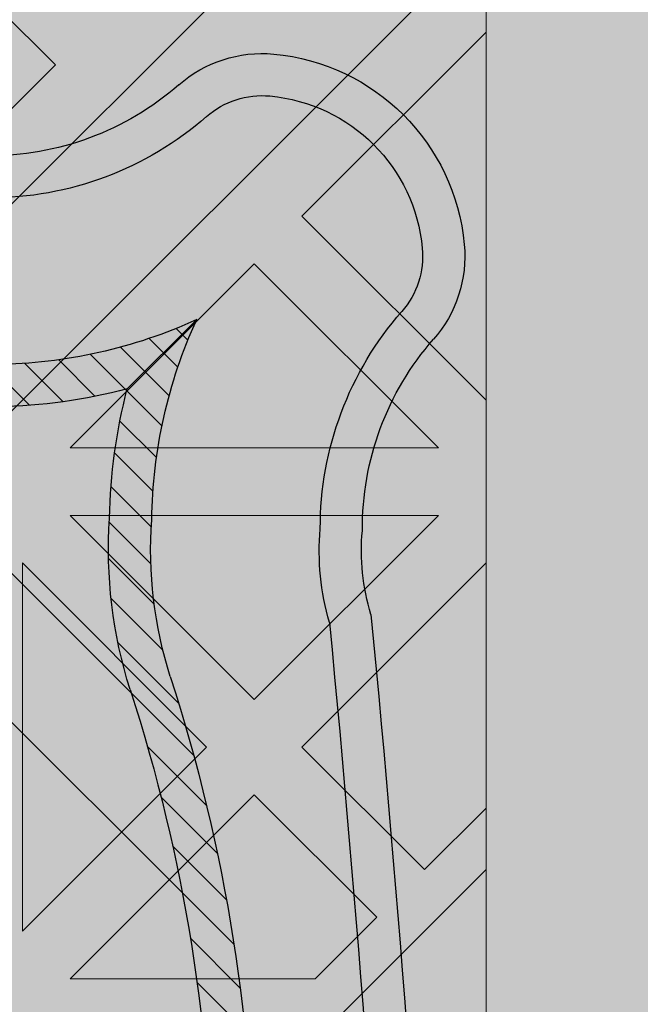
# Model space of a CAD drawing. Units: inches. Extents: x 844 to 2234, y 346 to 1084.
# Tile 39 of 93: x 1260.074 to 1262.421, y 701.353 to 705.079. Entities that reach past the tile are written whole.
import ezdxf

# ---------------------------------------------------------------- set-up
doc = ezdxf.new("R2010")
doc.units = ezdxf.units.IN
doc.header["$MEASUREMENT"] = 0
doc.layers.add('furniture', color=8, linetype='Continuous', lineweight=18)
doc.layers.add('RA-AP-01$0$INT', color=35, linetype='Continuous', lineweight=5)
doc.layers.add('RA-AP-01$0$FURN', color=3, linetype='Continuous')
doc.layers.add('RA-AP-01$0$WOOD', color=64, linetype='Continuous')

# ---------------------------------------------------------------- blocks, each defined once
blk = doc.blocks.new('A$C18D01794')
at = {"layer": 'RA-AP-01$0$INT'}
blk.add_hatch(color=256, dxfattribs=at).paths.add_polyline_path([(4.505206456958071, -7.906712009588039), (5.305206456958072, -7.906712009588039), (5.305206456958072, -7.106712009588038), (5.255206456951893, -7.106712009588036), (5.25520645694868, -7.856712009570104), (4.555206456959269, -7.856712009588616), (4.555206456956052, -7.106712009588038), (4.505206456958073, -7.106712009588038)])
h = blk.add_hatch(color=256, dxfattribs=at)
h.paths.add_polyline_path([(4.585917135068448, -7.856712009587804), (4.614201406330596, -7.856712009587056), (4.668846067270487, -7.802067348644738), (4.723490728212344, -7.856712009584164), (4.771774999457151, -7.856712009582887), (4.826419660396886, -7.80206734864072), (4.862780050090322, -7.838427738332541), (4.844495778842715, -7.856712009580965), (4.862780050090411, -7.856712009580482), (4.905206456960182, -7.814285602707865), (4.947632863832445, -7.856712009578238), (4.965917135079675, -7.856712009577755), (4.947632863831759, -7.838427738330656), (4.983993253523576, -7.802067348637219), (5.038637914464627, -7.856712009575829), (5.08692218571208, -7.856712009574554), (5.141566846649976, -7.802067348634224), (5.196211507589851, -7.856712009571666), (5.224495778822615, -7.856712009570916), (4.905206456953975, -7.537422687702283)])
h.paths.add_polyline_path([(4.895206456956031, -7.575706958950402), (4.895206456958921, -7.684996280828174), (4.840561796018589, -7.630351619890275)], flags=16)
h.paths.add_polyline_path([(4.915206456955638, -7.575706958949956), (4.969851117895509, -7.630351619887399), (4.915206456957609, -7.684996280827732)], flags=16)
h.paths.add_polyline_path([(4.826419660395175, -7.644493755514321), (4.881064321335613, -7.699138416452331), (4.771774999456703, -7.69913841645522)], flags=16)
h.paths.add_polyline_path([(4.983993253519558, -7.644493755510815), (5.038637914460456, -7.699138416449285), (4.929348592581548, -7.69913841645126)], flags=16)
h.paths.add_polyline_path([(4.881064321336025, -7.719138416452334), (4.826419660397532, -7.773783077393256), (4.771774999457062, -7.719138416455217)], flags=16)
h.paths.add_polyline_path([(4.929348592582019, -7.71913841645126), (5.038637914460982, -7.719138416449284), (4.983993253522945, -7.773783077389749)], flags=16)
h.paths.add_polyline_path([(4.895206456960191, -7.733280552075633), (4.895206456962115, -7.806001331460164), (4.876922185715016, -7.824285602708492), (4.840561796021581, -7.787925213016675)], flags=16)
h.paths.add_polyline_path([(4.915206456958487, -7.733280552075187), (4.969851117899527, -7.787925213013798), (4.933490728206909, -7.824285602708034), (4.9152064569598, -7.806001331461736)], flags=16)
h.paths.add_polyline_path([(4.757632863832376, -7.733280552079264), (4.812277524772842, -7.787925213017304), (4.757632863834348, -7.842569873958233)], flags=16)
h.paths.add_polyline_path([(4.737632863832376, -7.73328055207979), (4.737632863834348, -7.842569873958701), (4.682988202893906, -7.787925213020692)], flags=16)
h.paths.add_polyline_path([(5.05278005008503, -7.733280552072701), (5.052780050087917, -7.842569873951664), (4.998135389146995, -7.787925213013169)], flags=16)
h.paths.add_polyline_path([(5.072780050085024, -7.733280552072333), (5.127424711025931, -7.787925213010806), (5.072780050087916, -7.842569873951244)], flags=16)
h.paths.add_polyline_path([(4.935917135072783, -7.506712009583784), (5.255206456948811, -7.826001331459767), (5.255206456948932, -7.797717060211899), (5.200561796010279, -7.743072399273238), (5.255206456949403, -7.688427738334128), (5.25520645694961, -7.640143467086677), (5.200561796009787, -7.585498806146837), (5.236922185702417, -7.549138416454212), (5.255206456949919, -7.56742268770172), (5.255206456949998, -7.549138416454178), (5.212780050078687, -7.506712009583814), (5.25520645695036, -7.464285602712145), (5.255206456950438, -7.446001331464763), (5.236922185702424, -7.464285602712779), (5.200561796009796, -7.427925213020149), (5.255206456950753, -7.373280552079203), (5.25520645695096, -7.324996280834394), (5.200561796010322, -7.270351619893748), (5.255206456951428, -7.215706958952649), (5.255206456951547, -7.187422687705071)])
h.paths.add_polyline_path([(5.042988202883395, -7.42792521302065), (5.097632863823085, -7.373280552080975), (5.097632863822622, -7.482569873959883)], flags=16)
h.paths.add_polyline_path([(5.028846067259663, -7.442067348644384), (5.083490728198774, -7.496712009583504), (4.974201406321001, -7.496712009583035)], flags=16)
h.paths.add_polyline_path([(5.117632863823087, -7.37328055208089), (5.172277524762331, -7.42792521302015), (5.11763286382262, -7.482569873959851)], flags=16)
h.paths.add_polyline_path([(5.08349072819877, -7.516712009582191), (5.028846067259652, -7.571356670521302), (4.974201406320998, -7.516712009582638)], flags=16)
h.paths.add_polyline_path([(5.131774999446817, -7.35913841645716), (5.186419660386065, -7.413783077396415), (5.241064321325782, -7.359138416456712)], flags=17)
h.paths.add_polyline_path([(5.131774999446228, -7.496712009583703), (5.186419660386065, -7.442067348643883), (5.222780050079488, -7.478427738337313), (5.204495778832781, -7.496712009584014)], flags=16)
h.paths.add_polyline_path([(5.097632863822613, -7.530854145205813), (5.097632863823061, -7.640143467084723), (5.042988202883383, -7.585498806145032)], flags=16)
h.paths.add_polyline_path([(5.131774999446899, -7.339138416457162), (5.241064321325809, -7.339138416456712), (5.186419660386591, -7.284493755517479)], flags=17)
h.paths.add_polyline_path([(5.131774999446226, -7.516712009581999), (5.204495778830767, -7.516712009581702), (5.22278005007868, -7.534996280829206), (5.186419660386049, -7.571356670521828)], flags=16)
h.paths.add_polyline_path([(5.11763286382262, -7.530854145205852), (5.17227752476232, -7.585498806145562), (5.117632863823064, -7.64014346708481)], flags=16)
h.paths.add_polyline_path([(5.186419660386069, -7.599640941770585), (5.241064321325754, -7.654285602710281), (5.131774999446791, -7.654285602709814)], flags=16)
h.paths.add_polyline_path([(5.131774999446872, -7.674285602709813), (5.24106432132578, -7.674285602710282), (5.186419660386554, -7.728930263649504)], flags=16)
h.paths.add_polyline_path([(5.255206456951811, -7.126001331467467), (5.255206456951895, -7.106712009588038), (4.555206456956052, -7.106712009588038), (4.555206456956136, -7.12600133146746), (4.905206456953973, -7.476001331465289)])
h.paths.add_polyline_path([(4.983993253513404, -7.368930263651977), (4.92934859257295, -7.314285602713969), (5.03863791445186, -7.314285602711063)], flags=16)
h.paths.add_polyline_path([(4.969851117889988, -7.383072399276016), (4.915206456952556, -7.437717060215906), (4.915206456949648, -7.328427738338133)], flags=16)
h.paths.add_polyline_path([(4.929348592572535, -7.294285602713971), (4.983993253511019, -7.239640941773039), (5.038637914451496, -7.294285602711065)], flags=16)
h.paths.add_polyline_path([(5.052780050074912, -7.280143467087016), (4.998135389134438, -7.225498806148989), (5.052780050072919, -7.170854145208052)], flags=16)
h.paths.add_polyline_path([(5.07278005007491, -7.280143467086489), (5.072780050072918, -7.170854145207579), (5.127424711013374, -7.225498806145578)], flags=16)
h.paths.add_polyline_path([(4.89520645695295, -7.437717060216355), (4.840561796013067, -7.383072399278919), (4.895206456950961, -7.328427738338582)], flags=16)
h.paths.add_polyline_path([(4.915206456948365, -7.280143467090674), (4.915206456946434, -7.207422687704125), (4.933490728192729, -7.18913841645701), (4.969851117886972, -7.225498806149623)], flags=16)
h.paths.add_polyline_path([(4.881064321327021, -7.314285602715054), (4.82641966038902, -7.368930263655506), (4.771774999448108, -7.314285602717047)], flags=16)
h.paths.add_polyline_path([(4.895206456950073, -7.280143467091125), (4.840561796009022, -7.225498806152518), (4.876922185700835, -7.18913841645908), (4.895206456948749, -7.207422687706589)], flags=16)
h.paths.add_polyline_path([(4.983993253510392, -7.211356670525576), (4.947632863816944, -7.174996280833758), (4.965917135064043, -7.156712009585847), (5.038637914448995, -7.156712009584522)], flags=16)
h.paths.add_polyline_path([(4.881064321326543, -7.294285602715056), (4.771774999447578, -7.294285602717046), (4.826419660385607, -7.239640941776569)], flags=16)
h.paths.add_polyline_path([(4.905206456946447, -7.19913841645844), (4.862780050074785, -7.156712009587725), (4.947632863816685, -7.156712009586302)], flags=16)
h.paths.add_polyline_path([(5.14156684663679, -7.211356670521528), (5.086922185696452, -7.156712009583639), (5.196211507574223, -7.156712009581651)], flags=16)
h.paths.add_polyline_path([(4.8264196603837, -7.211356670529104), (4.771774999442643, -7.156712009590501), (4.8444957788276, -7.156712009588568), (4.862780050075511, -7.17499628083566)], flags=16)
h.paths.add_polyline_path([(4.812277524760289, -7.225498806153156), (4.757632863822258, -7.28014346709363), (4.757632863819352, -7.170854145214669)], flags=16)
h.paths.add_polyline_path([(4.73763286382226, -7.280143467093997), (4.682988202881349, -7.22549880615554), (4.737632863819352, -7.170854145215086)], flags=16)
h.paths.add_polyline_path([(4.723490728195188, -7.156712009591787), (4.668846067257299, -7.211356670532127), (4.614201406317417, -7.156712009594693)], flags=16)
h.paths.add_polyline_path([(4.597632863829262, -7.506712009583814), (4.555206456957951, -7.54913841645418), (4.555206456958029, -7.56742268770172), (4.573490728205535, -7.549138416454212), (4.609851117898167, -7.585498806146839), (4.555206456958338, -7.640143467086675), (4.555206456958546, -7.688427738334125), (4.60985111789767, -7.743072399273238), (4.555206456959015, -7.797717060211899), (4.555206456959138, -7.826001331459767), (4.874495778835167, -7.506712009583786), (4.5552064569564, -7.187422687705062), (4.555206456956523, -7.215706958952644), (4.609851117897629, -7.270351619893746), (4.555206456956988, -7.324996280834396), (4.555206456957198, -7.373280552079195), (4.609851117898153, -7.427925213020147), (4.573490728205528, -7.464285602712779), (4.555206456957507, -7.446001331464756), (4.555206456957585, -7.464285602712143)])
h.paths.add_polyline_path([(4.712780050085332, -7.482569873959882), (4.712780050084863, -7.373280552080972), (4.767424711024555, -7.42792521302065)], flags=16)
h.paths.add_polyline_path([(4.726922185709173, -7.496712009583504), (4.781566846648288, -7.442067348644384), (4.836211507586949, -7.496712009583033)], flags=16)
h.paths.add_polyline_path([(4.692780050085327, -7.482569873959851), (4.638135389145619, -7.427925213020149), (4.692780050084865, -7.373280552080892)], flags=16)
h.paths.add_polyline_path([(4.726922185709182, -7.516712009582191), (4.836211507586949, -7.51671200958264), (4.7815668466483, -7.571356670521304)], flags=16)
h.paths.add_polyline_path([(4.678637914461726, -7.496712009583706), (4.605917135075169, -7.496712009584014), (4.587632863828464, -7.478427738337311), (4.623993253521887, -7.442067348643881)], flags=16)
h.paths.add_polyline_path([(4.712780050085336, -7.530854145205816), (4.767424711024568, -7.585498806145034), (4.71278005008489, -7.640143467084724)], flags=16)
h.paths.add_polyline_path([(4.678637914461726, -7.516712009582001), (4.623993253521899, -7.571356670521829), (4.587632863829271, -7.534996280829206), (4.605917135077185, -7.5167120095817)], flags=16)
h.paths.add_polyline_path([(4.692780050085336, -7.530854145205848), (4.692780050084889, -7.64014346708481), (4.638135389145632, -7.585498806145562)], flags=16)
h.paths.add_polyline_path([(4.623993253521885, -7.413783077396415), (4.678637914461131, -7.359138416457161), (4.56934859258217, -7.359138416456712)], flags=17)
h.paths.add_polyline_path([(4.623993253521901, -7.599640941770568), (4.678637914461158, -7.654285602709814), (4.569348592582195, -7.654285602710281)], flags=16)
h.paths.add_polyline_path([(4.678637914461051, -7.339138416457162), (4.623993253521361, -7.284493755517479), (4.569348592582143, -7.339138416456712)], flags=17)
h.paths.add_polyline_path([(4.678637914461076, -7.674285602709813), (4.623993253521399, -7.728930263649504), (4.569348592582167, -7.674285602710281)], flags=16)
h = blk.add_hatch(color=256, dxfattribs=at)
h.paths.add_polyline_path([(4.905206456954232, -7.537422687702028), (4.874495778835232, -7.506712009583718), (4.555206456959138, -7.826001331459766), (4.555206456959269, -7.856712009588616), (4.585917135068449, -7.856712009587804)])
h.paths.add_polyline_path([(4.935917135072152, -7.506712009583152), (4.905206456953497, -7.537422687701806), (5.224495778822614, -7.856712009570917), (5.255206456948681, -7.856712009570104), (5.255206456948813, -7.826001331459768)])
h.paths.add_polyline_path([(5.255206456951549, -7.18742268770507), (5.255206456951813, -7.126001331467461), (4.905206456953563, -7.476001331465701), (4.935917135072559, -7.506712009584006)])
h.paths.add_polyline_path([(4.874495778835167, -7.506712009583785), (4.905206456953818, -7.476001331465132), (4.555206456956135, -7.126001331467458), (4.555206456956399, -7.187422687705064)])
h = blk.add_hatch(color=256, dxfattribs=at)
h.paths.add_polyline_path([(4.781566846647504, -7.442067348645805), (4.836211507586161, -7.496712009584463), (4.726922185708388, -7.496712009584918)])
h.paths.add_polyline_path([(4.836211507586161, -7.516712009584068), (4.781566846647504, -7.571356670522723), (4.726922185708388, -7.516712009583606)])
h.paths.add_polyline_path([(4.76742471102377, -7.585498806146453), (4.712780050084083, -7.640143467086137), (4.712780050084542, -7.530854145207227)])
h.paths.add_polyline_path([(4.692780050084544, -7.530854145207257), (4.692780050084084, -7.64014346708622), (4.638135389144834, -7.585498806146965)])
h.paths.add_polyline_path([(4.678637914460932, -7.516712009583407), (4.623993253521102, -7.571356670523233), (4.587632863827676, -7.53499628082981), (4.605917135074382, -7.516712009583104)])
h.paths.add_polyline_path([(4.573490728204743, -7.54913841645434), (4.60985111789737, -7.585498806146969), (4.555206456957541, -7.640143467086797), (4.555206456957237, -7.567422687701846)])
h.paths.add_polyline_path([(4.623993253521098, -7.599640941770699), (4.67863791446035, -7.654285602709951), (4.56934859258139, -7.654285602710407)])
h.paths.add_polyline_path([(4.678637914460275, -7.67428560270995), (4.623993253520583, -7.728930263649637), (4.56934859258136, -7.674285602710405)])
h.paths.add_polyline_path([(4.609851117896854, -7.743072399273369), (4.555206456958196, -7.797717060212026), (4.555206456957738, -7.688427738334254)])
h.paths.add_polyline_path([(4.597632863828475, -7.506712009583301), (4.555206456957283, -7.549138416454495), (4.555206456956805, -7.464285602712587)])
h.paths.add_polyline_path([(4.678637914460932, -7.496712009585113), (4.605917135076396, -7.496712009585417), (4.587632863828479, -7.478427738337913), (4.623993253521104, -7.442067348645284)])
h.paths.add_polyline_path([(4.692780050084091, -7.373280552082301), (4.692780050084548, -7.482569873961267), (4.638135389144834, -7.427925213021552)])
h.paths.add_polyline_path([(4.767424711023772, -7.427925213022072), (4.712780050084545, -7.48256987396129), (4.712780050084089, -7.373280552082384)])
h.paths.add_polyline_path([(4.67863791446036, -7.359138416457298), (4.623993253521105, -7.41378307739655), (4.569348592581399, -7.35913841645684)])
h.paths.add_polyline_path([(4.609851117897371, -7.427925213020278), (4.573490728204743, -7.464285602712907), (4.555206456957237, -7.446001331465401), (4.555206456957548, -7.373280552080448)])
h.paths.add_polyline_path([(4.623993253520596, -7.284493755517612), (4.67863791446028, -7.339138416457299), (4.569348592581367, -7.339138416456838)])
h.paths.add_polyline_path([(4.609851117896867, -7.270351619893878), (4.555206456957749, -7.324996280832994), (4.55520645695821, -7.21570695895522)])
h = blk.add_hatch(color=256, dxfattribs=at)
h.paths.add_polyline_path([(4.969851117891331, -7.630351619889621), (4.915206456952669, -7.575706958950966), (4.915206456952222, -7.684996280828739)])
h.paths.add_polyline_path([(4.895206456953064, -7.575706958950968), (4.840561796014413, -7.630351619889628), (4.895206456953533, -7.684996280828741)])
h.paths.add_polyline_path([(4.826419660390684, -7.644493755513362), (4.771774999451003, -7.699138416453052), (4.881064321329913, -7.699138416452587)])
h.paths.add_polyline_path([(4.881064321329884, -7.719138416452585), (4.771774999450921, -7.719138416453052), (4.82641966039018, -7.773783077392298)])
h.paths.add_polyline_path([(4.895206456953734, -7.733280552076196), (4.840561796013912, -7.787925213016031), (4.876922185707337, -7.824285602709455), (4.895206456954043, -7.806001331462747)])
h.paths.add_polyline_path([(4.862780050082808, -7.838427738332388), (4.826419660390178, -7.802067348639763), (4.771774999450351, -7.856712009579595), (4.844495778835303, -7.856712009579895)])
h.paths.add_polyline_path([(4.812277524766446, -7.787925213016036), (4.757632863827191, -7.733280552076788), (4.757632863826741, -7.842569873955747)])
h.paths.add_polyline_path([(4.737632863827191, -7.733280552076863), (4.682988202887508, -7.787925213016558), (4.737632863826743, -7.842569873955778)])
h.paths.add_polyline_path([(4.668846067263777, -7.802067348640287), (4.614201406325123, -7.856712009578949), (4.723490728202894, -7.856712009579402)])
h.paths.add_polyline_path([(4.905206456953846, -7.814285602708654), (4.862780050082654, -7.856712009579847), (4.947632863824561, -7.85671200958032)])
h.paths.add_polyline_path([(4.915206456952028, -7.733280552076195), (4.91520645695173, -7.806001331460731), (4.933490728199234, -7.824285602708648), (4.96985111789186, -7.787925213016022)])
h.paths.add_polyline_path([(5.038637914454841, -7.719138416453029), (4.929348592575874, -7.71913841645258), (4.983993253515593, -7.773783077392289)])
h.paths.add_polyline_path([(4.983993253515065, -7.644493755513352), (4.929348592575849, -7.699138416452582), (5.038637914454755, -7.699138416453031)])
h.paths.add_polyline_path([(5.052780050079843, -7.73328055207676), (4.998135389140595, -7.787925213016018), (5.052780050080309, -7.842569873955721)])
h.paths.add_polyline_path([(4.983993253516868, -7.802067348639752), (4.947632863824241, -7.838427738332383), (4.965917135071747, -7.856712009579888), (5.038637914456701, -7.856712009579572)])
h.paths.add_polyline_path([(5.127424711019533, -7.787925213016519), (5.072780050079843, -7.733280552076838), (5.07278005008031, -7.842569873955751)])
h.paths.add_polyline_path([(5.141566846643269, -7.802067348640248), (5.086922185704154, -7.85671200957937), (5.196211507581929, -7.856712009578901)])
for p, q in [((4.555206456956052, -7.106712009588036), (4.555206456959269, -7.856712009588616)), ((4.55520645695807, -7.464285602712626), (4.555206456957598, -7.549138416454534)), ((4.597632863829264, -7.506712009583814), (4.555206456957598, -7.549138416454534)), ((4.874495778835167, -7.506712009583786), (4.555206456959136, -7.826001331459769)), ((4.605917135074869, -7.516712009584017), (4.587632863829269, -7.534996280829206)), ((4.605917135076771, -7.5167120095817), (4.678637914461723, -7.516712009581999)), ((4.678637914461723, -7.516712009581999), (4.623993253521898, -7.571356670521829)), ((4.692780050085336, -7.530854145205847), (4.638135389145632, -7.585498806145562)), ((4.692780050084889, -7.64014346708481), (4.692780050085336, -7.530854145205847)), ((4.623993253521899, -7.571356670521829), (4.587632863829269, -7.534996280829206)), ((4.905206456953975, -7.537422687702283), (4.585917135071132, -7.856712009585121)), ((4.555206456958031, -7.56742268770172), (4.573490728205535, -7.549138416454212)), ((4.609851117898167, -7.585498806146839), (4.573490728205535, -7.549138416454214)), ((4.555206456958033, -7.56742268770172), (4.555206456958345, -7.640143467086671)), ((4.555206456958345, -7.640143467086671), (4.609851117898167, -7.585498806146837)), ((4.692780050084889, -7.64014346708481), (4.638135389145632, -7.585498806145562)), ((4.569348592582195, -7.654285602710281), (4.623993253521901, -7.599640941770568)), ((4.678637914461158, -7.654285602709814), (4.623993253521901, -7.599640941770568)), ((4.678637914461158, -7.654285602709814), (4.569348592582195, -7.654285602710281)), ((4.569348592582168, -7.674285602710281), (4.623993253521399, -7.728930263649504)), ((4.678637914461078, -7.674285602709813), (4.569348592582168, -7.674285602710281)), ((4.6239932535214, -7.728930263649502), (4.678637914461078, -7.674285602709813)), ((4.555206456958551, -7.68842773833413), (4.60985111789767, -7.743072399273238)), ((4.682988202893908, -7.78792521302069), (4.737632863832376, -7.733280552079792)), ((4.555206456959017, -7.797717060211899), (4.60985111789767, -7.743072399273238)), ((4.737632863834348, -7.842569873958701), (4.682988202893906, -7.787925213020692))]:
    blk.add_line(p, q, dxfattribs=at)
blk = doc.blocks.new('A$C32926AE1')
at = {"layer": 'RA-AP-01$0$WOOD'}
h = blk.add_hatch(color=256, dxfattribs=at)
h.dxf.hatch_style = 1
h.paths.add_polyline_path([(5.157430609644524, 4.573483066760929, -0.1009492694046607), (5.155401577623758, 4.593365984175333, -0.1842662638101597), (5.172249623284174, 4.638795604568598, 0.2056608120311276), (5.179560981299304, 4.661316324430096, 0.3614336704623542), (5.134352340494423, 4.706524965234944, 0.2056608120311297), (5.111831620632933, 4.699213607219793, -0.1842662638101113), (5.066402000239693, 4.682365561559342, -0.1055311479399994), (5.045656153913092, 4.68467289944697, 0.1567636581983829), (4.763886414745334, 4.684672899446966, -0.1055311479399895), (4.743140568418733, 4.68236556155934, -0.1842662638100833), (4.6977109480255, 4.69921360721979, 0.2056608120302612), (4.675190228164109, 4.706524965234949, 0.3614336704708441), (4.629981587358889, 4.66131632442871, 0.2056608120245944), (4.637292945374126, 4.638795604567974, -0.1842662638101024), (4.654140991034615, 4.59336598417475, -0.1009492694055169), (4.652111959013835, 4.573483066760181, 0.021410119221476), (4.629748025606143, 4.156712009541676, 0.0214101192214795), (4.652111959013809, 3.739940952323101, -0.1009492694059586), (4.654140991034615, 3.720058034908448, -0.1842662638100975), (4.637292945374126, 3.674628414515226, 0.2056608120245705), (4.629981587358889, 3.652107694654492, 0.3614336704708879), (4.675190228164113, 3.606899053848249, 0.2056608120302384), (4.697710948025501, 3.614210411863408, -0.1842662638100995), (4.743140568418738, 3.63105845752386, -0.1055311479402541), (4.763886414745388, 3.628751119636215, 0.1567636581983776), (5.045656153913137, 3.628751119636244, -0.1055311479397538), (5.066402000239692, 3.631058457523857, -0.1842662638101067), (5.111831620632931, 3.614210411863407, 0.2056608120310924), (5.134352340494417, 3.606899053848256, 0.3614336704624001), (5.179560981299307, 3.652107694653103, 0.2056608120311314), (5.172249623284175, 3.6746284145146, -0.1842662638101402), (5.155401577623758, 3.72005803490786, -0.1009492694051366), (5.15743060964455, 3.739940952322354, 0.0214101192215073), (5.179794543052287, 4.156712009541468, 0.0214101192215252)])
h.paths.add_polyline_path([(4.639748609479751, 4.156712009541513, 0.0213537860821624), (4.661970494867118, 3.741887061152232, -0.094075836301374), (4.664143710413708, 3.7196126951003, -0.1824818158568985), (4.644813765429836, 3.668037719127816, 0.2056608120245319), (4.639939526753007, 3.653023905887301, 0.3614336704710246), (4.676106439397173, 3.616856993242342, 0.2056608120302234), (4.691120252638095, 3.621731231919122, -0.1824818158602558), (4.742695228611606, 3.641061176902986, -0.1029891339458722), (4.766991894714349, 3.638256818950944, 0.156709409989566), (5.042550673941472, 3.638256818950105, -0.102989133958497), (5.066847340047078, 3.641061176902949, -0.1824818158594995), (5.118422316020358, 3.621731231919103, 0.2056608120311416), (5.133436129261316, 3.616856993242346, 0.3614336704621468), (5.169603041905217, 3.653023905886178, 0.2056608120310986), (5.164728803228477, 3.668037719127177, -0.1824818158565612), (5.145398858244737, 3.719612695099578, -0.0940758363009313), (5.147572073791232, 3.741887061151398, 0.0213537860822023), (5.169793959178681, 4.156712009541451, 0.0213537860822226), (5.147572073791203, 4.571536957931898, -0.0940758363005034), (5.145398858244737, 4.59381132398362, -0.1824818158565587), (5.164728803228476, 4.645386299956021, 0.2056608120311045), (5.169603041905216, 4.66040011319702, 0.3614336704621845), (5.133436129261313, 4.696567025840856, 0.2056608120310773), (5.118422316020359, 4.691692787164098, -0.182481815859508), (5.066847340047078, 4.67236284218025, -0.1029891339584606), (5.04255067394148, 4.675167200133092, 0.156709409989566), (4.766991894714357, 4.675167200132257, -0.1029891339458842), (4.742695228611611, 4.672362842180213, -0.1824818158602725), (4.691120252638095, 4.691692787164077, 0.2056608120302152), (4.676106439397174, 4.696567025840858, 0.3614336704710363), (4.639939526753005, 4.660400113195899, 0.2056608120245495), (4.644813765429837, 4.645386299955384, -0.1824818158568934), (4.664143710413708, 4.593811323982902, -0.0940758363009187), (4.661970494867149, 4.571536957931074, 0.021353786082177)], flags=16)
h.paths.add_polyline_path([(5.129794543052235, 4.432167055276933, -0.0141661062790638), (5.130152669293814, 4.156927903047693, -0.0141661062790647), (5.129794543052234, 3.881688750818433, -0.0785247771143638), (5.10979738006795, 3.755143611847103, 0.0945969212073497), (5.105408519571111, 3.717898134952927, 0.1043170707844957), (5.116074640131521, 3.670385395016088, 0.1043170707864965), (5.068561900193738, 3.681051515576561, 0.09459692119553), (5.031316423304057, 3.676662655080835, -0.1580239521427272), (4.778226145355827, 3.676662655080367, 0.0945969211986668), (4.740980668464973, 3.681051515576592, 0.1043170707882822), (4.693467928526415, 3.670385395015844, 0.1043170707867916), (4.704134049087309, 3.717898134953662, 0.0945969211972894), (4.69974518859162, 3.755143611844042, -0.0785247771163196), (4.679748025606343, 3.881688750818406, -0.0141661062790663), (4.679389899364763, 4.156927903047693, -0.0141661062790672), (4.679748025606343, 4.432167055276998, -0.0785247771163064), (4.699745188591625, 4.55871219425134, 0.094596921197333), (4.704134049087308, 4.595957671141738, 0.1043170707867205), (4.693467928526416, 4.643470411079523, 0.1043170707882628), (4.740980668464965, 4.632804290518776, 0.0945969211988114), (4.778226145355874, 4.637193151015016, -0.158023952142669), (5.031316423304015, 4.637193151014546, 0.0945969211956361), (5.068561900193736, 4.632804290518806, 0.1043170707864979), (5.11607464013152, 4.643470411079278, 0.1043170707844617), (5.105408519571112, 4.595957671142455, 0.0945969212074597), (5.109797380067959, 4.558712194248236, -0.0785247771143467)], flags=0)
h.paths.add_polyline_path([(5.119794532311105, 4.432259799204851, -0.0142000800617244), (5.120156169157484, 4.156927903047701, -0.0142000800617277), (5.119794532311105, 3.881596006890482, -0.0784894509520253), (5.100273383573699, 3.758192358677797, 0.0940138827242913), (5.095413455884425, 3.717477693979438, 0.0606271852308753), (5.099615656341024, 3.686844378806616, 0.0606271852322524), (5.068982341167493, 3.691046579263239, 0.0940138827010453), (5.028267676478798, 3.686186651576848, -0.1580706864508061), (4.781274892180912, 3.686186651576435, 0.0940138827026903), (4.740560227491556, 3.691046579263279, 0.0606271852339895), (4.709926912317155, 3.686844378806508, 0.0606271852329405), (4.714129112773991, 3.717477693980356, 0.094013882701304), (4.709269185087677, 3.758192358669163, -0.0784894509577193), (4.689748036347473, 3.881596006890469, -0.014200080061729), (4.689386399501094, 4.156927903047709, -0.0142000800617217), (4.689748036347473, 4.432259799204808, -0.078489450957724), (4.709269185087651, 4.555663447426125, 0.0940138827014585), (4.714129112773992, 4.596378112114996, 0.0606271852329731), (4.709926912317154, 4.62701142728886, 0.0606271852340196), (4.74056022749157, 4.622809226832087, 0.0940138827024997), (4.781274892180847, 4.627669154518912, -0.1580706864508359), (5.028267676478777, 4.627669154518526, 0.0940138827010946), (5.068982341167492, 4.622809226832129, 0.060627185232254), (5.099615656341024, 4.627011427288751, 0.0606271852308727), (5.095413455884425, 4.59637811211593, 0.0940138827241088), (5.100273383573675, 4.555663447417647, -0.0784894509520978)], flags=0)
h.paths.add_polyline_path([(5.06978912287499, 4.430218106756144, -0.014241683694547), (5.070173729147532, 4.156927903047672, -0.0142416836945458), (5.06978912287499, 3.883637699339223, -0.0800609523125196), (5.052662118612511, 3.773463122773442, 0.0526421978001116), (5.04590916754064, 3.740550867606997, 0.0526421977992423), (5.012996912374707, 3.73379791653534, -0.1583028414718258), (4.796545656286308, 3.73379791653451, 0.0526421978034211), (4.763633401117837, 3.740550867607021, 0.0526421978018622), (4.756880450045755, 3.773463122774558, -0.0800609523117106), (4.739753445783639, 3.883637699339268, -0.0142416836945435), (4.739368839511098, 4.156927903047671, -0.0142416836945477), (4.739753445783639, 4.430218106756155, -0.0800609523116345), (4.75688045004574, 4.540392683320762, 0.052642197801941), (4.763633401117837, 4.573304938488346, 0.0526421978035071), (4.796545656286361, 4.580057889560873, -0.1583028414717561), (5.012996912374669, 4.580057889560039, 0.0526421977993048), (5.04590916754064, 4.57330493848837, 0.0526421978002057), (5.052662118612529, 4.540392683321868, -0.080060952312477)], flags=0)
h.paths.add_polyline_path([(5.049789715110557, 4.43038092723357, -0.0143097550741839), (5.05018085590259, 4.156927903047715, -0.0143097550741854), (5.049789715110558, 3.883474878861827, -0.0800685599149176), (5.03362098255317, 3.779581877367999, 0.0306258898956367), (5.028241146483733, 3.758218888663947, 0.0306258898977031), (5.006878157778253, 3.75283905259408, -0.1583983521624096), (4.802664410878162, 3.752839052594731, 0.0306258898946014), (4.781301422174808, 3.758218888663924, 0.0306258898967912), (4.775921586105202, 3.779581877368794, -0.080068559914251), (4.759752853548071, 3.883474878861786, -0.0143097550741854), (4.759361712756037, 4.156927903047671, -0.0143097550741854), (4.759752853548071, 4.430380927233557, -0.0800685599142479), (4.775921586105193, 4.534273928726546, 0.0306258898968306), (4.781301422174808, 4.555636917431444, 0.0306258898945754), (4.802664410878143, 4.561016753500631, -0.1583983521624168), (5.006878157778244, 4.561016753501291, 0.0306258898977177), (5.028241146483733, 4.555636917431421, 0.0306258898958182), (5.03362098255321, 4.534273928727244, -0.080068559914796)], flags=0)
h.paths.add_polyline_path([(4.999766070382627, 4.428171244713864, -0.0143443147609634), (5.000198441819402, 4.156927903047689, -0.0143443147609612), (4.999766070382627, 3.885684561381556, -0.0784641635803329), (4.987356730658798, 3.799103304488872, -0.1506053783831347), (4.822185837999821, 3.79910330448882, -0.0784641635803318), (4.809776498276007, 3.885684561381509, -0.014344314760963), (4.809344126839227, 4.156927903047677, -0.0143443147609645), (4.809776498276007, 4.428171244713873, -0.0784641635803192), (4.822185837999822, 4.514752501606549, -0.1506053783831338), (4.987356730658798, 4.514752501606494, -0.078464163580285)], flags=0)
h.paths.add_polyline_path([(4.979755254238824, 4.42764379880488, -0.0143772539198268), (4.980205517789977, 4.156927903047693, -0.0143772539198275), (4.979755254238824, 3.886212007290489, -0.0689242507424422), (4.971183264704897, 3.815276770442801, -0.1296645318904179), (4.838359303953726, 3.815276770442746, -0.0689242507424186), (4.829787314419809, 3.886212007290419, -0.0143772539198292), (4.829337050868653, 4.156927903047653, -0.0143772539198325), (4.829787314419809, 4.427643798804946, -0.0689242507424211), (4.838359303953725, 4.498579035652621, -0.1296645318904187), (4.971183264704897, 4.498579035652565, -0.0689242507424401)], flags=0)
h = blk.add_hatch(color=256, dxfattribs=at)
h.dxf.hatch_style = 1
h.paths.add_polyline_path([(5.145398858244737, 4.59381132398362, -0.1824818158565616), (5.164728803228476, 4.645386299956021, 0.2056608120311045), (5.169603041905216, 4.66040011319702, 0.3614336704621845), (5.133436129261313, 4.696567025840856, 0.2056608120310773), (5.118422316020359, 4.691692787164098, -0.182481815859508), (5.066847340047078, 4.67236284218025, -0.1029891339584606), (5.04255067394148, 4.675167200133092, 0.156709409989566), (4.766991894714357, 4.675167200132257, -0.1029891339458842), (4.742695228611611, 4.672362842180213, -0.1824818158602725), (4.691120252638095, 4.691692787164077, 0.2056608120302152), (4.676106439397174, 4.696567025840858, 0.3614336704710363), (4.639939526753005, 4.660400113195899, 0.2056608120245495), (4.644813765429837, 4.645386299955384, -0.1824818158568934), (4.664143710413708, 4.593811323982902, -0.0940758363009187), (4.661970494867149, 4.571536957931074, 0.0213537860821772), (4.639748609479751, 4.156712009541507, 0.0213537860821625), (4.661970494867119, 3.741887061152226, -0.0940758363013071), (4.664143710413708, 3.719612695100309, -0.1824818158569294), (4.644813765429836, 3.668037719127816, 0.2056608120245319), (4.639939526753007, 3.653023905887301, 0.3614336704710246), (4.676106439397173, 3.616856993242342, 0.2056608120302234), (4.691120252638095, 3.621731231919122, -0.1824818158602558), (4.742695228611606, 3.641061176902986, -0.1029891339458722), (4.766991894714349, 3.638256818950944, 0.156709409989566), (5.042550673941472, 3.638256818950105, -0.102989133958497), (5.066847340047078, 3.641061176902949, -0.1824818158594995), (5.118422316020358, 3.621731231919103, 0.2056608120311416), (5.133436129261316, 3.616856993242346, 0.3614336704621468), (5.169603041905217, 3.653023905886178, 0.2056608120310986), (5.164728803228477, 3.668037719127177, -0.1824818158565612), (5.145398858244737, 3.719612695099578, -0.0940758363009313), (5.147572073791232, 3.741887061151398, 0.0213537860822023), (5.169793959178681, 4.156712009541451, 0.0213537860822226), (5.147572073791203, 4.571536957931898, -0.0940758363004996)])
h.paths.add_polyline_path([(5.109797380067958, 4.55871219424824, -0.0785247771143472), (5.129794543052234, 4.432167055276936, -0.0141661062790644), (5.130152669293814, 4.156927903047685, -0.014166106279066), (5.129794543052234, 3.881688750818401, -0.0785247771143517), (5.109797380067946, 3.755143611847092, 0.0945969212073132), (5.105408519571111, 3.717898134952929, 0.1043170707844995), (5.116074640131521, 3.670385395016088, 0.1043170707864965), (5.068561900193738, 3.681051515576561, 0.09459692119553), (5.031316423304057, 3.676662655080835, -0.1580239521427272), (4.778226145355827, 3.676662655080367, 0.0945969211986668), (4.740980668464973, 3.681051515576592, 0.1043170707882822), (4.693467928526415, 3.670385395015844, 0.1043170707867916), (4.704134049087309, 3.717898134953662, 0.0945969211972894), (4.69974518859162, 3.755143611844042, -0.0785247771163196), (4.679748025606343, 3.881688750818406, -0.0141661062790663), (4.679389899364763, 4.156927903047693, -0.0141661062790672), (4.679748025606343, 4.432167055276998, -0.0785247771163064), (4.699745188591625, 4.55871219425134, 0.094596921197333), (4.704134049087308, 4.595957671141738, 0.1043170707867205), (4.693467928526416, 4.643470411079523, 0.1043170707882628), (4.740980668464965, 4.632804290518776, 0.0945969211988114), (4.778226145355874, 4.637193151015016, -0.158023952142669), (5.031316423304015, 4.637193151014546, 0.0945969211956361), (5.068561900193736, 4.632804290518806, 0.1043170707864979), (5.11607464013152, 4.643470411079278, 0.1043170707844617), (5.105408519571112, 4.595957671142455, 0.0945969212074504)], flags=16)
h.paths.add_polyline_path([(5.100273383573655, 4.55566344741771, -0.0784894509521388), (5.119794532311105, 4.432259799204852, -0.0142000800617252), (5.120156169157484, 4.156927903047686, -0.014200080061726), (5.119794532311105, 3.881596006890502, -0.0784894509520446), (5.100273383573696, 3.758192358677786, 0.0940138827242721), (5.095413455884425, 3.717477693979436, 0.0606271852308692), (5.099615656341024, 3.686844378806616, 0.0606271852322522), (5.068982341167493, 3.691046579263239, 0.0940138827010453), (5.028267676478798, 3.686186651576848, -0.1580706864508061), (4.781274892180912, 3.686186651576435, 0.0940138827026903), (4.740560227491556, 3.691046579263279, 0.0606271852339895), (4.709926912317155, 3.686844378806508, 0.0606271852329405), (4.714129112773991, 3.717477693980356, 0.094013882701304), (4.709269185087677, 3.758192358669163, -0.0784894509577193), (4.689748036347473, 3.881596006890469, -0.014200080061729), (4.689386399501094, 4.156927903047709, -0.0142000800617217), (4.689748036347473, 4.432259799204808, -0.078489450957724), (4.709269185087651, 4.555663447426125, 0.0940138827014585), (4.714129112773992, 4.596378112114996, 0.0606271852329731), (4.709926912317154, 4.62701142728886, 0.0606271852340196), (4.74056022749157, 4.622809226832087, 0.0940138827024997), (4.781274892180847, 4.627669154518912, -0.1580706864508359), (5.028267676478777, 4.627669154518526, 0.0940138827010946), (5.068982341167492, 4.622809226832129, 0.060627185232254), (5.099615656341024, 4.627011427288751, 0.0606271852308727), (5.095413455884425, 4.59637811211593, 0.094013882723957)], flags=0)
h.paths.add_polyline_path([(5.04590916754064, 4.57330493848837, 0.0526421978002057), (5.052662118612529, 4.540392683321868, -0.0800609523124783), (5.06978912287499, 4.430218106756142, -0.0142416836945469), (5.070173729147532, 4.156927903047672, -0.0142416836945458), (5.06978912287499, 3.883637699339223, -0.0800609523125196), (5.052662118612511, 3.773463122773442, 0.0526421978001116), (5.04590916754064, 3.740550867606997, 0.0526421977992423), (5.012996912374707, 3.73379791653534, -0.1583028414718258), (4.796545656286308, 3.73379791653451, 0.0526421978034211), (4.763633401117837, 3.740550867607021, 0.0526421978018622), (4.756880450045755, 3.773463122774558, -0.0800609523117106), (4.739753445783639, 3.883637699339268, -0.0142416836945435), (4.739368839511098, 4.156927903047671, -0.0142416836945477), (4.739753445783639, 4.430218106756155, -0.0800609523116345), (4.75688045004574, 4.540392683320762, 0.052642197801941), (4.763633401117837, 4.573304938488346, 0.0526421978035071), (4.796545656286361, 4.580057889560873, -0.1583028414717561), (5.012996912374669, 4.580057889560039, 0.0526421977993048)], flags=0)
h.paths.add_polyline_path([(5.028241146483733, 4.555636917431422, 0.0306258898956949), (5.033620982553182, 4.534273928727329, -0.0800685599148649), (5.049789715110557, 4.430380927233569, -0.0143097550741839), (5.05018085590259, 4.156927903047715, -0.0143097550741854), (5.049789715110558, 3.883474878861827, -0.0800685599149176), (5.03362098255317, 3.779581877367999, 0.0306258898956367), (5.028241146483733, 3.758218888663947, 0.0306258898977031), (5.006878157778253, 3.75283905259408, -0.1583983521624096), (4.802664410878162, 3.752839052594731, 0.0306258898946014), (4.781301422174808, 3.758218888663924, 0.0306258898967912), (4.775921586105202, 3.779581877368794, -0.080068559914251), (4.759752853548071, 3.883474878861786, -0.0143097550741854), (4.759361712756037, 4.156927903047671, -0.0143097550741854), (4.759752853548071, 4.430380927233557, -0.0800685599142479), (4.775921586105193, 4.534273928726546, 0.0306258898968306), (4.781301422174808, 4.555636917431444, 0.0306258898945754), (4.802664410878143, 4.561016753500631, -0.1583983521624168), (5.006878157778244, 4.561016753501291, 0.0306258898977174)], flags=0)
h.paths.add_polyline_path([(4.987356730658798, 4.514752501606494, -0.0784641635803018), (4.999766070382627, 4.428171244713845, -0.0143443147609637), (5.000198441819402, 4.156927903047665, -0.0143443147609622), (4.999766070382628, 3.885684561381514, -0.0784641635802952), (4.987356730658797, 3.799103304488872, -0.1506053783831338), (4.822185837999821, 3.799103304488819, -0.0784641635803342), (4.809776498276007, 3.885684561381512, -0.0143443147609628), (4.809344126839227, 4.156927903047676, -0.0143443147609646), (4.809776498276007, 4.428171244713873, -0.0784641635803192), (4.822185837999822, 4.514752501606549, -0.1506053783831338)], flags=0)
h.paths.add_polyline_path([(4.971183264704897, 4.498579035652566, -0.0689242507424384), (4.979755254238824, 4.427643798804883, -0.0143772539198276), (4.980205517789977, 4.15692790304768, -0.0143772539198258), (4.979755254238823, 3.88621200729051, -0.0689242507424628), (4.971183264704897, 3.815276770442801, -0.129664531890417), (4.838359303953726, 3.815276770442746, -0.0689242507424186), (4.829787314419809, 3.886212007290419, -0.0143772539198292), (4.829337050868653, 4.156927903047653, -0.0143772539198325), (4.829787314419809, 4.427643798804946, -0.0689242507424211), (4.838359303953725, 4.498579035652621, -0.1296645318904187)], flags=0)
h = blk.add_hatch(dxfattribs=at)
h.set_pattern_fill('ANSI31', color=256, scale=0.05, style=0)
h.set_pattern_definition([(45, (0, 0), (-0.0044194173824159, 0.0044194173824159), [])])
h.paths.add_polyline_path([(5.130152669293814, 4.156927903047704, 0.0141661062790657), (5.129794543052234, 4.432167055276982, 0.0777827904001433), (5.110168979996553, 4.557559993161921, -0.0976515123401879), (5.105408519571111, 4.595957671142454, -0.1043170707844687), (5.116074640131522, 4.64347041107928), (5.099615656341024, 4.627011427288751, 0.0606271852308727), (5.095413455884425, 4.59637811211593, 0.0940138827241088), (5.100273383573675, 4.555663447417647, -0.0784894509520972), (5.119794532311105, 4.432259799204852, -0.0142000800617252), (5.120156169157484, 4.156927903047686, -0.014200080061726), (5.119794532311105, 3.881596006890502, -0.0784894509520446), (5.100273383573696, 3.758192358677786, 0.0940138827242721), (5.095413455884425, 3.717477693979436, 0.0606271852308692), (5.099615656341024, 3.686844378806616), (5.116074640131519, 3.67038539501609, -0.1043170707844594), (5.105408519571112, 3.717898134952912, -0.0976515123401594), (5.11016897999655, 3.756295812933435, 0.0777827904001654), (5.129794543052234, 3.881688750818409, 0.0141661062790665)])
h.paths.add_polyline_path([(5.030164222210597, 3.676291055149937, -0.0976515123472002), (5.068561900193739, 3.681051515576561, -0.1043170707864927), (5.116074640131521, 3.670385395016088), (5.099615656341024, 3.686844378806616, 0.0606271852322522), (5.068982341167493, 3.691046579263239, 0.0940138827010453), (5.028267676478798, 3.686186651576848, -0.1580706864508061), (4.781274892180912, 3.686186651576435, 0.0940138827026903), (4.740560227491556, 3.691046579263279, 0.0606271852339913), (4.709926912317154, 3.686844378806508), (4.693467928526416, 3.670385395015845, -0.1043170707882796), (4.740980668464973, 3.681051515576592, -0.0976515123427246), (4.779378346446416, 3.676291055150394, 0.156512506893803)])
h.paths.add_polyline_path([(4.689748036347473, 3.881596006890472, -0.014200080061729), (4.689386399501094, 4.156927903047712, -0.0142000800617195), (4.689748036347473, 4.432259799204768, -0.078489450957742), (4.709269185087648, 4.555663447426114, 0.0940138827014821), (4.714129112773992, 4.596378112114995, 0.0606271852329748), (4.709926912317154, 4.62701142728886), (4.693467928526414, 4.643470411079524, -0.1043170707867939), (4.704134049087309, 4.595957671141706, -0.09765151234893), (4.699373588660725, 4.557559993157876, 0.0777827903975372), (4.679748025606343, 4.432167055276987, 0.0141661062790675), (4.679389899364763, 4.156927903047675, 0.0141661062790641), (4.679748025606343, 3.88168875081843, 0.0777827903975637), (4.699373588660724, 3.756295812937497, -0.0976515123490278), (4.704134049087308, 3.717898134953629, -0.1043170707867196), (4.693467928526416, 3.670385395015845), (4.709926912317155, 3.686844378806508, 0.0606271852329413), (4.714129112773991, 3.717477693980357, 0.0940138827013084), (4.709269185087676, 3.758192358669166, -0.0784894509577192)])
h.paths.add_polyline_path([(4.779378346446434, 4.63756475094498, -0.0976515123427943), (4.740980668464964, 4.632804290518776, -0.1043170707882609), (4.693467928526416, 4.643470411079523), (4.709926912317154, 4.62701142728886, 0.0606271852340196), (4.74056022749157, 4.622809226832087, 0.0940138827024997), (4.781274892180847, 4.627669154518912, -0.1580706864508359), (5.028267676478777, 4.627669154518526, 0.0940138827010946), (5.068982341167492, 4.622809226832129, 0.060627185232254), (5.099615656341024, 4.627011427288751), (5.116074640131521, 4.643470411079279, -0.1043170707865022), (5.068561900193735, 4.632804290518806, -0.0976515123475899), (5.030164222210446, 4.637564750945479, 0.1565125068936924)])
h = blk.add_hatch(dxfattribs=at)
h.set_pattern_fill('ANSI32', color=256, scale=0.2, style=0)
h.set_pattern_definition([(45, (0, 0), (-0.0530330085889911, 0.0530330085889911), []), (45, (0.035355339, 0), (-0.0530330085889911, 0.0530330085889911), [])])
h.paths.add_polyline_path([(5.119794532311105, 4.432259799204823, 0.0777015974868765), (5.10065834347252, 4.554469821747928, -0.0968902511992216), (5.095413455884425, 4.596378112115931, -0.060627185230871), (5.099615656341024, 4.627011427288751, -0.060627185232254), (5.068982341167492, 4.622809226832129, -0.0968902512198245), (5.027074050790956, 4.628054114423209, 0.1564657949319105), (4.782468517866163, 4.628054114422785, -0.0968902512152247), (4.740560227491555, 4.622809226832088, -0.0606271852339878), (4.709926912317155, 4.627011427288859, -0.0606271852329413), (4.714129112773991, 4.596378112115011, -0.0968902512205338), (4.708884225182929, 4.554469821738175, 0.0777015974804443), (4.689748036347473, 4.43225979920482, 0.0142000800617215), (4.689386399501094, 4.156927903047726, 0.0142000800617273), (4.689748036347473, 3.88159600689052, 0.077701597480541), (4.708884225182985, 3.759385984357019, -0.096890251220082), (4.714129112773992, 3.717477693980371, -0.0606271852329731), (4.709926912317154, 3.686844378806507, -0.060627185233988), (4.740560227491554, 3.691046579263279, -0.0968902512152569), (4.782468517866175, 3.685801691672578, 0.1564657949319236), (5.027074050790988, 3.685801691672169, -0.0968902512197451), (5.068982341167491, 3.691046579263239, -0.0606271852322557), (5.099615656341024, 3.686844378806616, -0.0606271852308727), (5.095413455884425, 3.717477693979438, -0.0968902511991229), (5.100658343472507, 3.7593859843474, 0.0777015974868745), (5.119794532311105, 3.8815960068905, 0.014200080061726), (5.120156169157484, 4.156927903047685, 0.0142000800617238)])
h.paths.add_polyline_path([(5.070173729147531, 4.156927903047684, -0.0142416836945481), (5.06978912287499, 3.883637699339191, -0.0800609523125107), (5.052662118612505, 3.773463122773424, 0.0526421978000811), (5.04590916754064, 3.740550867606997, 0.0526421977993214), (5.012996912374658, 3.733797916535325, -0.1583028414717916), (4.796545656286304, 3.733797916534512, 0.0526421978034138), (4.763633401117837, 3.740550867607021, 0.0526421978018622), (4.756880450045755, 3.773463122774558, -0.0800609523117106), (4.739753445783639, 3.883637699339268, -0.0142416836945435), (4.739368839511098, 4.156927903047671, -0.0142416836945477), (4.739753445783639, 4.430218106756155, -0.0800609523116345), (4.75688045004574, 4.540392683320762, 0.052642197801941), (4.763633401117837, 4.573304938488346, 0.0526421978035071), (4.796545656286361, 4.580057889560873, -0.1583028414717561), (5.012996912374669, 4.580057889560039, 0.0526421977993048), (5.04590916754064, 4.57330493848837, 0.0526421978002057), (5.052662118612529, 4.540392683321868, -0.0800609523124783), (5.06978912287499, 4.430218106756142, -0.0142416836945463)], flags=16)
h.paths.add_polyline_path([(5.050180855902591, 4.156927903047686, -0.0143097550741856), (5.049789715110558, 3.883474878861795, -0.0800685599148126), (5.033620982553202, 3.7795818773681, 0.0306258898957837), (5.028241146483733, 3.758218888663947, 0.0306258898977031), (5.006878157778253, 3.75283905259408, -0.1583983521624096), (4.802664410878162, 3.752839052594731, 0.0306258898946014), (4.781301422174808, 3.758218888663924, 0.0306258898967912), (4.775921586105202, 3.779581877368794, -0.080068559914251), (4.759752853548071, 3.883474878861786, -0.0143097550741854), (4.759361712756037, 4.156927903047671, -0.0143097550741854), (4.759752853548071, 4.430380927233557, -0.0800685599142479), (4.775921586105193, 4.534273928726546, 0.0306258898968306), (4.781301422174808, 4.555636917431444, 0.0306258898945754), (4.802664410878143, 4.561016753500631, -0.1583983521624168), (5.006878157778244, 4.561016753501291, 0.0306258898977177), (5.028241146483733, 4.555636917431421, 0.0306258898958182), (5.03362098255321, 4.534273928727244, -0.0800685599147973), (5.049789715110557, 4.430380927233568, -0.0143097550741854)], flags=0)
h.paths.add_polyline_path([(5.000198441819402, 4.15692790304769, -0.0143443147609622), (4.999766070382627, 3.885684561381539, -0.0784641635803169), (4.987356730658798, 3.799103304488873, -0.1506053783831347), (4.822185837999821, 3.79910330448882, -0.0784641635803318), (4.809776498276007, 3.885684561381509, -0.014344314760963), (4.809344126839227, 4.156927903047677, -0.0143443147609645), (4.809776498276007, 4.428171244713873, -0.0784641635803192), (4.822185837999822, 4.514752501606549, -0.1506053783831338), (4.987356730658798, 4.514752501606494, -0.0784641635803018), (4.999766070382627, 4.428171244713845, -0.0143443147609624)], flags=0)
h.paths.add_polyline_path([(4.980205517789976, 4.156927903047707, -0.0143772539198295), (4.979755254238824, 3.886212007290466, -0.06892425074242), (4.971183264704897, 3.815276770442801, -0.129664531890417), (4.838359303953726, 3.815276770442746, -0.0689242507424186), (4.829787314419809, 3.886212007290419, -0.0143772539198292), (4.829337050868653, 4.156927903047653, -0.0143772539198325), (4.829787314419809, 4.427643798804946, -0.0689242507424211), (4.838359303953725, 4.498579035652621, -0.1296645318904187), (4.971183264704897, 4.498579035652565, -0.0689242507424418), (4.979755254238824, 4.427643798804878, -0.0143772539198259)], flags=0)
blk.add_line((4.709926912317154, 4.62701142728886), (4.693467928526416, 4.643470411079523), dxfattribs=at)
blk.add_line((4.709926912317154, 4.62701142728886), (4.693467928526416, 4.643470411079523), dxfattribs=at)
for centre, radius, start, end in [((4.679771284329349, 4.656735268264593), 0.0499999999998897, 95.25687599443106, 174.7431240064049), ((4.67793886186326, 4.676651147052671), 0.0299999999999992, 48.77105092035662, 95.25687599427984), ((4.742507915094499, 4.750332633143934), 0.0679700159630274, 228.7710509203537, 270.5333070513671), ((4.679771284329334, 4.656735268264609), 0.0399999999998732, 95.25687599445018, 174.7431240064249), ((4.67793886186326, 4.676651147052671), 0.0199999999999984, 48.77105092035742, 95.25687599428184), ((4.742507915094546, 4.750332633143919), 0.0779700159630467, 228.7710509203206, 270.1376463011373), ((4.659855405541232, 4.658567690730234), 0.0300000000000005, 174.7431240062535, 221.2289490796905), ((4.65985540554127, 4.658567690730245), 0.0200000000000369, 174.7431240062188, 221.2289490796444), ((4.586173919450017, 4.593998637498934), 0.077970015963029, 359.8623536996133, 41.22894907969008), ((4.586173919450015, 4.5944304245111), 0.1179700159630316, 0.7417751874182703, 24.56332695026347), ((4.742507915094493, 4.750764420156106), 0.1179700159630538, 245.436673049926, 269.258224813113), ((4.586173919450019, 4.593998637498935), 0.0679700159630267, 359.4666929486785, 41.22894907969187), ((4.586173919450018, 4.594430424511101), 0.1279700159630281, 0.8720682535796656, 14.74980897308237), ((4.742507915094622, 4.750764420156106), 0.1279700159630606, 255.250191027056, 269.1279317467988), ((4.604388392048166, 4.588829985554355), 0.1000000000000129, 342.4716349543535, 4.087328884225124), ((4.604388392048173, 4.588829985554312), 0.1099999999999923, 342.4514408378524, 3.934690089293226), ((4.604388392048149, 4.588398198542093), 0.0500000000000008, 342.6443160247905, 5.702070765404379), ((4.604388392048171, 4.58839819854224), 0.060000000000024, 343.6788686696151, 5.176192161067998), ((9.505218788282013, 4.104079819130551), 4.875754844654793, 174.47541031816, 179.3814986516462), ((9.505218788282013, 4.104079819130551), 4.865754844654794, 174.4870438419329, 179.3814986516462), ((5.090145208887515, 4.432167055276791), 0.4103971832811724, 162.0403002448777, 179.9999999999736), ((5.090145208887515, 4.432167055276791), 0.4003971832811724, 162.0403002448777, 179.9999999999736)]:
    blk.add_arc(centre, radius, start, end, dxfattribs=at)
blk = doc.blocks.new('A$C5D2F253E')
at = {"layer": 'RA-AP-01$0$FURN', "xscale": -0.7999999999883585, "yscale": 0.7999999999883585, "zscale": 0.8, "rotation": 90}
blk.add_blockref('A$C18D01794', (-5.687757199772477, 4.75791982714071), dxfattribs=at)
at = {"layer": 'RA-AP-01$0$WOOD', "rotation": 270}
blk.add_blockref('A$C32926AE1', (-4.161339601644158, 5.73852594588169), dxfattribs=at)

msp = doc.modelspace()

# ---------------------------------------------------------------- block references
at = {"layer": 'furniture', "xscale": -15.94108302203742, "yscale": 15.94108302203742, "zscale": 15.94108302203742, "rotation": 270}
msp.add_blockref('A$C5D2F253E', (1244.08405109492, 696.2584716700112), dxfattribs=at)

doc.saveas('drawing.dxf')
